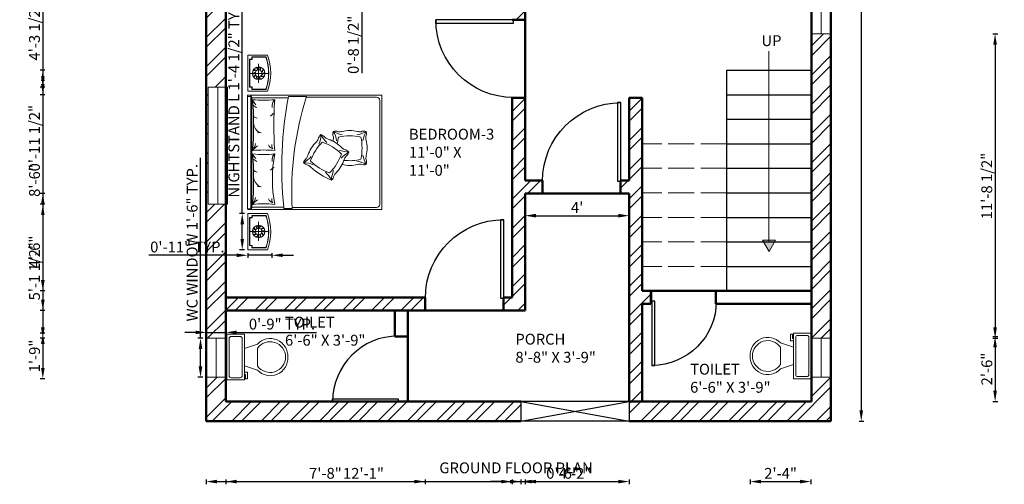
# Model space of a CAD drawing. Units: inches. Extents: x -83 to 371, y -457 to 76.
# Tile 1 of 4: x -83 to 371, y -457 to -243. Entities that reach past the tile are written whole.
import ezdxf

# ---------------------------------------------------------------- set-up
doc = ezdxf.new("R2010")
doc.units = ezdxf.units.IN
doc.linetypes.add('ACAD_ISO02W100', pattern=[15, 12, -3])
for name, color, linetype, lineweight in [('A-ANNO-DIMS', 2, 'Continuous', 18), ('A-ANNO-SYMB', 7, 'Continuous', 18), ('A-ANNO-TEXT', 7, 'Continuous', 25), ('A-AREA-IDEN', 7, 'Continuous', 25), ('A-DOOR', 3, 'Continuous', 25), ('A-FLOR-FIXT', 9, 'Continuous', 18), ('A-FLOR-STRS', 7, 'Continuous', 25), ('A-FLOR-STRS-OVHD', 8, 'ACAD_ISO02W100', 18), ('A-GLAZ', 4, 'Continuous', 18), ('A-WALL', 7, 'Continuous', 50), ('A-WALL-PATT', 252, 'Continuous', 13), ('furn', 28, 'Continuous', 18)]:
    doc.layers.add(name, color=color, linetype=linetype, lineweight=lineweight)
doc.styles.get("Standard").update_dxf_attribs({"font": 'arial.ttf'})
doc.dimstyles.new('ISO-25', dxfattribs={"dimtxt": 5, "dimasz": 5, "dimexe": 1.25, "dimexo": 0.625, "dimtad": 1, "dimlunit": 3, "dimtxsty": 'Standard', "dimcen": 2.5, "dimadec": 0, "dimazin": 0, "dimtfac": 1, "dimtmove": 0, "dimatfit": 3, "dimfxl": 1, "dimfxlon": 1, "dimarcsym": 0})

# ---------------------------------------------------------------- blocks, each defined once
blk = doc.blocks.new('*U2')
for p, q in [((9.5, -6), (9.5, -2)), ((-10, -8.5), (-8, -8.5)), ((-10, -9.5), (-10, -8.5)), ((-8, -8.5), (-8, -8)), ((-7, -8), (-7, -9.5)), ((-4, -8), (-6, -14)), ((4, -8), (6, -14)), ((-7, -9.5), (-10, -9.5)), ((4, -14), (-4, -14))]:
    blk.add_line(p, q)
blk.add_lwpolyline([(10.5, -8), (10.5, 0), (-10.5, 0), (-10.5, -8)], close=True)
for points in [[(-9.5, -2), (-9.5, -6)], [(8.5, -1), (-8.5, -1)], [(-8.5, -7), (8.5, -7)]]:
    blk.add_lwpolyline(points)
for centre, radius, start, end in [((-8.625, -1.875), 0.8839, 81.8699, 188.1301), ((8.625, -1.875), 0.8839, 351.8699, 98.1301), ((-8.625, -6.125), 0.8839, 171.869898, 278.1301), ((8.625, -6.125), 0.8839, 261.8699, 8.1301), ((-0.4772, -19.9188), 8.0953, 133.01722, 273.38), ((0.0374, -19.8731), 7.127, 124.50543, 269.7), ((-0.0373, -19.8731), 7.127, 270.3, 55.4946), ((0.4773, -19.9188), 8.0953, 266.62, 46.9828)]:
    blk.add_arc(centre, radius, start, end)
blk = doc.blocks.new('*U4')
for p, q in [((0, 0), (0, -6)), ((40, 0), (40, -6))]:
    blk.add_line(p, q)
blk.add_lwpolyline([(0, 0), (0, 40), (1.75, 40), (1.75, 0)], close=True)
blk.add_arc((0, 0), 40, 0, 90)
blk = doc.blocks.new('*D7')
at = {"layer": 'A-ANNO-DIMS', "color": 0, "lineweight": -2, "transparency": 16777216}
for p, q in [((149.97, -332.63), (149.97, -334.88)), ((154.97, -333.63), (192.97, -333.63)), ((197.97, -332.63), (197.97, -334.88))]:
    blk.add_line(p, q, dxfattribs=at)
at = {"layer": 'A-ANNO-DIMS', "color": 0, "transparency": 16777216}
for points in [[(154.97, -332.79), (154.97, -334.46), (149.97, -333.63)], [(192.97, -332.79), (192.97, -334.46), (197.97, -333.63)]]:
    blk.add_solid(points, dxfattribs=at)
at = {"layer": 'Defpoints', "color": 0, "transparency": 16777216}
for p in [(149.97, -331.2), (197.97, -331.2), (197.97, -333.63)]:
    blk.add_point(p, dxfattribs=at)
at = {"layer": 'A-ANNO-DIMS', "color": 0, "transparency": 16777216, "insert": (173.97, -330.5), "char_height": 5, "attachment_point": 5}
blk.add_mtext("4'", dxfattribs=at)
blk = doc.blocks.new('*D9')
at = {"layer": 'A-ANNO-DIMS', "color": 0, "lineweight": -2, "transparency": 16777216}
for p, q in [((303.95, 15.68), (306.2, 15.68)), ((304.95, 10.68), (304.95, -423.32)), ((303.95, -428.32), (306.2, -428.32))]:
    blk.add_line(p, q, dxfattribs=at)
at = {"layer": 'A-ANNO-DIMS', "color": 0, "transparency": 16777216}
for points in [[(304.12, 10.68), (305.78, 10.68), (304.95, 15.68)], [(304.12, -423.32), (305.78, -423.32), (304.95, -428.32)]]:
    blk.add_solid(points, dxfattribs=at)
at = {"layer": 'Defpoints', "color": 0, "transparency": 16777216}
for p in [(295.93, 15.68), (290.97, -428.32), (304.95, -428.32)]:
    blk.add_point(p, dxfattribs=at)
at = {"layer": 'A-ANNO-DIMS', "color": 0, "transparency": 16777216, "insert": (301.77, -206.32), "char_height": 5, "attachment_point": 5, "rotation": 90}
blk.add_mtext("37'", dxfattribs=at)
blk = doc.blocks.new('BED-DOUBLE')
for p, q in [((0.91, 59.91), (51.75, 59.91)), ((1.17, 60.37), (1.17, 45.16)), ((51.46, 60.37), (51.46, 43.19))]:
    blk.add_line(p, q)
for points in [[(0, 61.8), (0, 0), (52.66, 0), (52.66, 61.8)], [(52.17, 61.8), (52.17, 60.37), (0.3, 60.37), (0.3, 61.8), (52.66, 61.8)]]:
    blk.add_lwpolyline(points)
for points in [[(2.33, 49.32, 0.058596), (2.33, 59.5, 0.036889), (25.64, 59.5, 0.052163), (25.64, 49.32, 0.093111)], [(27.16, 49.32, 0.058596), (27.16, 59.5, 0.036648), (50.62, 59.5, 0.052163), (50.62, 49.32, 0.036967)], [(0.46, 45.16), (1.17, 45.16, -0.072944), (52.17, 43.04), (52.17, 34.6, 0.092568), (0.46, 41.29)]]:
    blk.add_lwpolyline(points, format="xyb", close=True)
for points in [[(0.91, 41.32), (0.91, 2.43, 0.414214), (2.43, 0.91), (50.23, 0.91, 0.414214), (51.75, 2.43), (51.75, 34.75)], [(16.91, 24, 0.111006), (25.6, 18.59, 0.119549), (31.09, 27.39, 0.107813), (22.42, 32.82)], [(22.37, 32.81, 0.121865), (16.91, 24, 0.121865)], [(20.68, 31.62, 0.091296), (21.61, 36.08, 0.091296), (24.41, 32.49, 0.091296)], [(26.47, 15.11, 0.159461), (27.65, 17.2, -0.076283), (28.59, 18.51, 0.115075), (32.41, 24.64, -0.076283), (33.17, 26.05, 0.159461), (34.52, 28.03)], [(30.07, 28.97, 0.091296), (34.52, 28.03, 0.091296), (30.93, 25.24, 0.091296)], [(18.01, 22.22, 0.091296), (13.56, 23.16, 0.091296), (17.15, 25.96, 0.091296)], [(23.17, 9.62, 0.111006), (33.41, 9.63, 0.119549), (33.41, 19.99, 0.033212), (30.26, 20.47)], [(27.4, 19.57, 0.091296), (26.47, 15.11, 0.091296), (23.67, 18.7)], [(31.71, 20.79, 0.091296), (35.99, 22.35, 0.091296), (34.42, 18.08, 0.091296)], [(35.99, 7.13, 0.159461), (35.88, 9.53, -0.076283), (35.99, 11.13, 0.115075), (35.99, 18.36, -0.076283), (35.88, 19.96, 0.159461), (35.99, 22.35)], [(25.05, 8.69, 0.091296), (20.77, 7.13, 0.091296), (22.34, 11.41, 0.091296)], [(34.42, 11.41, 0.091296), (35.99, 7.13, 0.091296), (31.71, 8.69)]]:
    blk.add_lwpolyline(points, format="xyb")
for centre, radius, start, end in [((0.91, 60.83), 0.913, 180, 270), ((7.74, 68), 10.08, 237.5379, 257.5233), ((-5.29, 49.98), 12.19, 36.4935, 51.2792), ((15.48, 53.46), 5.64, 96.6849, 148.3182), ((21.18, 56.67), 3.96, 141.8174, 169.8987), ((26.19, 56.11), 4.26, 130.5354, 160.3558), ((28.84, 52.52), 7.67, 114.6457, 134.1585), ((19.53, 49.98), 12.19, 36.4935, 51.2792), ((32.57, 68), 10.08, 237.5379, 257.5233), ((40.3, 53.46), 5.64, 96.6849, 148.3182), ((46.01, 56.67), 3.96, 141.8174, 169.8987), ((51.01, 56.11), 4.26, 130.5354, 160.3558), ((53.67, 52.52), 7.67, 114.6457, 134.1585), ((51.75, 60.83), 0.913, 270, 0), ((8.15, 56.6), 2.53, 335.8927, 16.1192), ((32.98, 56.6), 2.53, 335.8927, 16.1192), ((6.34, 49.09), 3.38, 114.2916, 160.9896), ((4.59, 48.38), 2.31, 76.4823, 128.5563), ((9.19, 42.25), 12.71, 36.2085, 45.0849), ((18.6, 49.75), 0.853, 353.7543, 77.2187), ((22.67, 46.41), 4.16, 44.406, 96.8342), ((23.45, 47.86), 2.64, 33.6349, 90.8456), ((31.17, 49.09), 3.38, 114.2916, 160.9896), ((29.41, 48.38), 2.31, 76.4823, 128.5563), ((34.02, 42.25), 12.71, 36.2085, 45.0849), ((43.42, 49.75), 0.853, 353.7543, 77.2187), ((47.5, 46.41), 4.16, 44.406, 96.8342), ((48.27, 47.86), 2.64, 33.6349, 90.8456), ((44.41, 10.55), 33.33, 138.3818, 157.7644), ((15.72, 36.39), 5.29, 315.5854, 333.0343), ((24.21, 33.23), 3.86, 132.4658, 168.7065), ((20.58, 32.5), 3.72, 37.2937, 74.0973), ((26.71, 38.99), 5.29, 233.2983, 250.7472), ((19.89, 18.93), 15.91, 45.1307, 71.3884), ((34.79, 33.99), 5.29, 225.7718, 243.2208), ((31.77, 25.77), 3.56, 39.4726, 79.6505), ((16.39, 25.78), 3.86, 222.6522, 258.8929), ((13.27, 17.27), 5.29, 45.7718, 63.2208), ((28.18, 32.33), 15.91, 225.1307, 251.3884), ((36.26, 14.74), 15.91, 166.8711, 193.1289), ((28.38, 6.89), 15.91, 77.0576, 78.7033), ((33.07, 27.55), 5.29, 257.6988, 275.1477), ((34.85, 18.98), 3.56, 71.3996, 111.5774), ((44.1, 14.85), 21.58, 173.1956, 194.0284), ((21.36, 12.27), 5.29, 53.2983, 70.7472), ((27.96, 19.27), 4.41, 218.7754, 250.3571), ((24.48, 8.17), 3.86, 159.3666, 195.6073), ((15.61, 9.99), 5.29, 355.0387, 12.4877), ((21.79, 10.85), 3.86, 254.5791, 290.8198), ((23.64, 1.98), 5.29, 77.6988, 95.1477), ((28.33, 22.65), 15.91, 257.0576, 283.3153), ((33.15, 2.01), 5.29, 85.2252, 102.6741), ((35.05, 11.45), 4.41, 250.7023, 282.284)]:
    blk.add_arc(centre, radius, start, end)
blk = doc.blocks.new('NIGHTSTAND-L')
for p, q in [((8.46, 1.22), (8.46, 10)), ((4.07, 5.61), (12.85, 5.61))]:
    blk.add_line(p, q)
blk.add_lwpolyline([(0, 1.52), (0, 10.65), (16.74, 10.65), (16.74, 1.52, -0.181818)], format="xyb", close=True)
for points in [[(1.92, 9.74), (1.92, 8.74), (0.91, 8.74)], [(2.01, 9.74), (2.01, 8.65), (0.91, 8.65)], [(1.92, 9.74), (14.83, 9.74)], [(1.92, 9.65), (14.83, 9.65)], [(14.73, 9.74), (14.73, 8.65), (15.83, 8.65)], [(14.83, 9.74), (14.83, 8.74), (15.83, 8.74)]]:
    blk.add_lwpolyline(points)
for points in [[(15.83, 8.74), (15.83, 2.16, -0.167087), (0.91, 2.16), (0.91, 8.74)], [(15.74, 8.74), (15.74, 2.22, -0.165559), (1, 2.22), (1, 8.74)]]:
    blk.add_lwpolyline(points, format="xyb")
for radius in [2.87, 1.55]:
    blk.add_circle((8.46, 5.61), radius)
for centre, radius, start, end in [((6.48, 6.34), 1.41, 232.3002, 292.538), ((6.49, 6.52), 1.84, 244.17, 290.4897), ((7.4, 7.5), 1.84, 208.17, 254.4897), ((7.28, 7.36), 1.41, 196.3002, 256.538), ((8.71, 7.76), 1.84, 172.17, 218.4897), ((8.53, 7.72), 1.41, 160.3002, 220.538), ((9.93, 7.2), 1.84, 136.17, 182.4897), ((9.76, 7.27), 1.41, 124.3002, 184.538), ((10.58, 6.04), 1.84, 100.17, 146.4897), ((10.49, 6.19), 1.41, 88.3002, 148.538), ((8.2, 3.47), 1.84, 352.17, 38.4897), ((10.42, 4.71), 1.84, 64.17, 110.4897), ((10.44, 4.89), 1.41, 52.3002, 112.538), ((9.64, 3.86), 1.41, 16.3002, 76.538), ((9.52, 3.73), 1.84, 28.17, 74.4897), ((6.43, 5.03), 1.41, 268.3002, 328.538), ((6.34, 5.19), 1.84, 280.17, 326.4897), ((7.16, 3.95), 1.41, 304.3002, 4.538), ((6.99, 4.02), 1.84, 316.17, 2.4897), ((8.38, 3.51), 1.41, 340.3002, 40.538)]:
    blk.add_arc(centre, radius, start, end)
blk = doc.blocks.new('NIGHTSTAND-R')
for p, q in [((8.28, 1.22), (8.28, 10)), ((12.67, 5.61), (3.89, 5.61))]:
    blk.add_line(p, q)
blk.add_lwpolyline([(16.74, 1.52), (16.74, 10.65), (0, 10.65), (0, 1.52, 0.181818)], format="xyb", close=True)
for points in [[(1.92, 9.74), (1.92, 8.74), (0.91, 8.74)], [(2.01, 9.74), (2.01, 8.65), (0.91, 8.65)], [(14.82, 9.74), (1.92, 9.74)], [(14.82, 9.65), (1.92, 9.65)], [(14.73, 9.74), (14.73, 8.65), (15.83, 8.65)], [(14.82, 9.74), (14.82, 8.74), (15.83, 8.74)]]:
    blk.add_lwpolyline(points)
for points in [[(0.91, 8.74), (0.91, 2.16, 0.167087), (15.83, 2.16), (15.83, 8.74)], [(1, 8.74), (1, 2.22, 0.165559), (15.74, 2.22), (15.74, 8.74)]]:
    blk.add_lwpolyline(points, format="xyb")
for radius in [2.87, 1.55]:
    blk.add_circle((8.28, 5.61), radius)
for centre, radius, start, end in [((6.3, 4.89), 1.41, 67.462, 127.6998), ((6.32, 4.7), 1.84, 69.5103, 115.83), ((7.23, 3.72), 1.84, 105.5103, 151.83), ((7.11, 3.86), 1.41, 103.462, 163.6998), ((6.26, 6.19), 1.41, 31.462, 91.6998), ((6.16, 6.03), 1.84, 33.5103, 79.83), ((8.54, 3.46), 1.84, 141.5103, 187.83), ((6.99, 7.27), 1.41, 355.462, 55.6998), ((6.82, 7.2), 1.84, 357.5103, 43.83), ((8.21, 7.72), 1.41, 319.462, 19.6998), ((8.24, 7.84), 1.84, 321.5103, 7.83), ((10.46, 6.59), 1.84, 249.5103, 295.83), ((10.48, 6.41), 1.41, 247.462, 307.6998), ((9.67, 7.44), 1.41, 283.462, 343.6998), ((9.55, 7.58), 1.84, 285.5103, 331.83), ((8.36, 3.5), 1.41, 139.462, 199.6998), ((9.75, 4.02), 1.84, 177.5103, 223.83), ((9.58, 3.95), 1.41, 175.462, 235.6998), ((10.41, 5.19), 1.84, 213.5103, 259.83), ((10.31, 5.03), 1.41, 211.462, 271.6998)]:
    blk.add_arc(centre, radius, start, end)
blk = doc.blocks.new('WIN-54IN')
blk.add_line((4.5, 54), (4.5, 0))
blk.add_lwpolyline([(0, 54), (9, 54), (9, 0), (0, 0)], close=True)
blk = doc.blocks.new('WIN-18IN')
blk.add_line((4.5, 18), (4.5, 0))
blk.add_lwpolyline([(0, 18), (9, 18), (9, 0), (0, 0)], close=True)
blk = doc.blocks.new('*D20')
at = {"layer": 'A-ANNO-DIMS', "color": 0, "lineweight": -2, "transparency": 16777216}
for p, q in [((0.34, -390.13), (0.34, -307.03)), ((1.34, -390.13), (-0.91, -390.13)), ((0.34, -403.13), (0.34, -395.13)), ((1.34, -408.13), (-0.91, -408.13))]:
    blk.add_line(p, q, dxfattribs=at)
at = {"layer": 'A-ANNO-DIMS', "color": 0, "transparency": 16777216}
for points in [[(-0.5, -395.13), (1.17, -395.13), (0.34, -390.13)], [(-0.5, -403.13), (1.17, -403.13), (0.34, -408.13)]]:
    blk.add_solid(points, dxfattribs=at)
at = {"layer": 'Defpoints', "color": 0, "transparency": 16777216}
for p in [(0.34, -390.13), (3.04, -390.13), (3.04, -408.13)]:
    blk.add_point(p, dxfattribs=at)
at = {"layer": 'A-ANNO-DIMS', "color": 0, "transparency": 16777216, "insert": (-2.87, -346.08), "char_height": 5, "attachment_point": 5, "rotation": 90}
blk.add_mtext('WC WINDOW 1\'-6" TYP.', dxfattribs=at)
blk = doc.blocks.new('*D21')
at = {"layer": 'A-ANNO-DIMS', "color": 0, "lineweight": -2, "transparency": 16777216}
for p, q in [((-1.96, -387.43), (-6.96, -387.43)), ((3.04, -388.43), (3.04, -386.18)), ((3.04, -387.43), (12.04, -387.43)), ((12.04, -388.43), (12.04, -386.18)), ((17.04, -387.43), (53.76, -387.43))]:
    blk.add_line(p, q, dxfattribs=at)
at = {"layer": 'A-ANNO-DIMS', "color": 0, "transparency": 16777216}
for points in [[(-1.96, -386.59), (-1.96, -388.26), (3.04, -387.43)], [(17.04, -386.59), (17.04, -388.26), (12.04, -387.43)]]:
    blk.add_solid(points, dxfattribs=at)
at = {"layer": 'Defpoints', "color": 0, "transparency": 16777216}
for p in [(3.04, -390.13), (12.04, -387.43), (12.04, -390.13)]:
    blk.add_point(p, dxfattribs=at)
at = {"layer": 'A-ANNO-DIMS', "color": 0, "transparency": 16777216, "insert": (37.9, -384.25), "char_height": 5, "attachment_point": 5}
blk.add_mtext('0\'-9" TYP.', dxfattribs=at)
blk = doc.blocks.new('*D24')
at = {"layer": 'A-ANNO-DIMS', "color": 0, "lineweight": -2, "transparency": 16777216}
for p, q in [((19.57, -332.63), (19.57, -231.32)), ((20.57, -332.63), (18.32, -332.63)), ((19.57, -344.37), (19.57, -337.63)), ((20.57, -349.37), (18.32, -349.37))]:
    blk.add_line(p, q, dxfattribs=at)
at = {"layer": 'A-ANNO-DIMS', "color": 0, "transparency": 16777216}
for points in [[(18.74, -337.63), (20.4, -337.63), (19.57, -332.63)], [(18.74, -344.37), (20.4, -344.37), (19.57, -349.37)]]:
    blk.add_solid(points, dxfattribs=at)
at = {"layer": 'Defpoints', "color": 0, "transparency": 16777216}
for p in [(19.57, -332.63), (22.08, -332.63), (22.08, -349.37)]:
    blk.add_point(p, dxfattribs=at)
at = {"layer": 'A-ANNO-DIMS', "color": 0, "transparency": 16777216, "insert": (16.36, -279.48), "char_height": 5, "attachment_point": 5, "rotation": 90}
blk.add_mtext('NIGHTSTAND L 1\'-4 1/2" TYP.', dxfattribs=at)
blk = doc.blocks.new('*D25')
at = {"layer": 'A-ANNO-DIMS', "color": 0, "lineweight": -2, "transparency": 16777216}
for p, q in [((17.08, -351.88), (-23.53, -351.88)), ((22.08, -350.88), (22.08, -353.13)), ((33.24, -351.88), (22.08, -351.88)), ((33.24, -350.88), (33.24, -353.13)), ((38.24, -351.88), (43.24, -351.88))]:
    blk.add_line(p, q, dxfattribs=at)
at = {"layer": 'A-ANNO-DIMS', "color": 0, "transparency": 16777216}
for points in [[(17.08, -351.05), (17.08, -352.71), (22.08, -351.88)], [(38.24, -351.05), (38.24, -352.71), (33.24, -351.88)]]:
    blk.add_solid(points, dxfattribs=at)
at = {"layer": 'Defpoints', "color": 0, "transparency": 16777216}
for p in [(22.08, -349.37), (33.24, -349.37), (22.08, -351.88)]:
    blk.add_point(p, dxfattribs=at)
at = {"layer": 'A-ANNO-DIMS', "color": 0, "transparency": 16777216, "insert": (-5.72, -348.7), "char_height": 5, "attachment_point": 5}
blk.add_mtext('0\'-11" TYP.', dxfattribs=at)
blk = doc.blocks.new('*D37')
at = {"layer": 'A-ANNO-DIMS', "color": 0, "lineweight": -2, "transparency": 16777216}
for p, q in [((74.66, -218.28), (74.66, -213.28)), ((73.66, -223.28), (75.91, -223.28)), ((74.66, -223.28), (74.66, -231.78)), ((73.66, -231.78), (75.91, -231.78)), ((74.66, -236.78), (74.66, -267.97))]:
    blk.add_line(p, q, dxfattribs=at)
at = {"layer": 'A-ANNO-DIMS', "color": 0, "transparency": 16777216}
for points in [[(73.83, -218.28), (75.5, -218.28), (74.66, -223.28)], [(73.83, -236.78), (75.5, -236.78), (74.66, -231.78)]]:
    blk.add_solid(points, dxfattribs=at)
at = {"layer": 'Defpoints', "color": 0, "transparency": 16777216}
for p in [(72.86, -223.28), (72.86, -231.78), (74.66, -231.78)]:
    blk.add_point(p, dxfattribs=at)
at = {"layer": 'A-ANNO-DIMS', "color": 0, "transparency": 16777216, "insert": (71.45, -254.88), "char_height": 5, "attachment_point": 5, "rotation": 90}
blk.add_mtext('0\'-8 1/2"', dxfattribs=at)
blk = doc.blocks.new('*D40')
at = {"layer": 'A-ANNO-DIMS', "color": 0, "lineweight": -2, "transparency": 16777216}
for p, q in [((-71.36, -222.99), (-73.61, -222.99)), ((-72.36, -227.99), (-72.36, -269.39)), ((-71.36, -274.39), (-73.61, -274.39))]:
    blk.add_line(p, q, dxfattribs=at)
at = {"layer": 'A-ANNO-DIMS', "color": 0, "transparency": 16777216}
for points in [[(-73.19, -227.99), (-71.52, -227.99), (-72.36, -222.99)], [(-73.19, -269.39), (-71.52, -269.39), (-72.36, -274.39)]]:
    blk.add_solid(points, dxfattribs=at)
at = {"layer": 'Defpoints', "color": 0, "transparency": 16777216}
for p in [(3.06, -222.99), (-72.36, -274.39), (3.85, -274.39)]:
    blk.add_point(p, dxfattribs=at)
at = {"layer": 'A-ANNO-DIMS', "color": 0, "transparency": 16777216, "insert": (-75.57, -248.69), "char_height": 5, "attachment_point": 5, "rotation": 90}
blk.add_mtext('4\'-3 1/2"', dxfattribs=at)
blk = doc.blocks.new('*D41')
at = {"layer": 'A-ANNO-DIMS', "color": 0, "lineweight": -2, "transparency": 16777216}
for p, q in [((-71.36, -328.39), (-73.61, -328.39)), ((-72.36, -333.39), (-72.36, -385.13)), ((-71.36, -390.13), (-73.61, -390.13))]:
    blk.add_line(p, q, dxfattribs=at)
at = {"layer": 'A-ANNO-DIMS', "color": 0, "transparency": 16777216}
for points in [[(-73.19, -333.39), (-71.52, -333.39), (-72.36, -328.39)], [(-73.19, -385.13), (-71.52, -385.13), (-72.36, -390.13)]]:
    blk.add_solid(points, dxfattribs=at)
at = {"layer": 'Defpoints', "color": 0, "transparency": 16777216}
for p in [(3.85, -328.39), (-72.36, -390.13), (3.04, -390.13)]:
    blk.add_point(p, dxfattribs=at)
at = {"layer": 'A-ANNO-DIMS', "color": 0, "transparency": 16777216, "insert": (-75.57, -359.26), "char_height": 5, "attachment_point": 5, "rotation": 90}
blk.add_mtext('5\'-1 1/2"', dxfattribs=at)
blk = doc.blocks.new('*D44')
at = {"layer": 'A-ANNO-DIMS', "color": 0, "lineweight": -2, "transparency": 16777216}
for p, q in [((365.66, -249.79), (367.91, -249.79)), ((366.66, -254.79), (366.66, -385.13)), ((365.66, -390.13), (367.91, -390.13))]:
    blk.add_line(p, q, dxfattribs=at)
at = {"layer": 'A-ANNO-DIMS', "color": 0, "transparency": 16777216}
for points in [[(365.83, -254.79), (367.49, -254.79), (366.66, -249.79)], [(365.83, -385.13), (367.49, -385.13), (366.66, -390.13)]]:
    blk.add_solid(points, dxfattribs=at)
at = {"layer": 'Defpoints', "color": 0, "transparency": 16777216}
for p in [(290.97, -249.79), (290.97, -390.13), (366.66, -390.13)]:
    blk.add_point(p, dxfattribs=at)
at = {"layer": 'A-ANNO-DIMS', "color": 0, "transparency": 16777216, "insert": (363.45, -319.96), "char_height": 5, "attachment_point": 5, "rotation": 90}
blk.add_mtext('11\'-8 1/2"', dxfattribs=at)
blk = doc.blocks.new('*D45')
at = {"layer": 'A-ANNO-DIMS', "color": 0, "lineweight": -2, "transparency": 16777216}
for p, q in [((138.97, -456.2), (133.97, -456.2)), ((143.97, -455.2), (143.97, -457.45)), ((143.97, -456.2), (149.97, -456.2)), ((149.97, -455.2), (149.97, -457.45)), ((154.97, -456.2), (174.51, -456.2))]:
    blk.add_line(p, q, dxfattribs=at)
at = {"layer": 'A-ANNO-DIMS', "color": 0, "transparency": 16777216}
for points in [[(138.97, -455.37), (138.97, -457.03), (143.97, -456.2)], [(154.97, -455.37), (154.97, -457.03), (149.97, -456.2)]]:
    blk.add_solid(points, dxfattribs=at)
at = {"layer": 'Defpoints', "color": 0, "transparency": 16777216}
for p in [(143.97, 6.68), (149.97, 6.68), (149.97, -456.2)]:
    blk.add_point(p, dxfattribs=at)
at = {"layer": 'A-ANNO-DIMS', "color": 0, "transparency": 16777216, "insert": (167.24, -453.02), "char_height": 5, "attachment_point": 5}
blk.add_mtext('0\'-6"', dxfattribs=at)
blk = doc.blocks.new('*D48')
at = {"layer": 'A-ANNO-DIMS', "color": 0, "lineweight": -2, "transparency": 16777216}
for p, q in [((242.97, 39.58), (242.97, 41.83)), ((281.97, 39.58), (281.97, 41.83)), ((247.97, 40.58), (276.97, 40.58))]:
    blk.add_line(p, q, dxfattribs=at)
at = {"layer": 'A-ANNO-DIMS', "color": 0, "transparency": 16777216}
for points in [[(247.97, 41.41), (247.97, 39.74), (242.97, 40.58)], [(276.97, 41.41), (276.97, 39.74), (281.97, 40.58)]]:
    blk.add_solid(points, dxfattribs=at)
at = {"layer": 'Defpoints', "color": 0, "transparency": 16777216}
for p in [(281.97, 40.58), (242.97, -266.56), (281.97, -266.56)]:
    blk.add_point(p, dxfattribs=at)
at = {"layer": 'A-ANNO-DIMS', "color": 0, "transparency": 16777216, "insert": (262.47, 43.75), "char_height": 5, "attachment_point": 5}
blk.add_mtext('3\'-3"', dxfattribs=at)
blk = doc.blocks.new('*D49')
at = {"layer": 'A-ANNO-DIMS', "color": 0, "lineweight": -2, "transparency": 16777216}
for p, q in [((-71.36, -266.56), (-73.61, -266.56)), ((-72.36, -271.56), (-72.36, -272.87)), ((-71.36, -277.87), (-73.61, -277.87)), ((-72.36, -277.87), (-72.36, -312.95))]:
    blk.add_line(p, q, dxfattribs=at)
at = {"layer": 'A-ANNO-DIMS', "color": 0, "transparency": 16777216}
for points in [[(-73.19, -271.56), (-71.52, -271.56), (-72.36, -266.56)], [(-73.19, -272.87), (-71.52, -272.87), (-72.36, -277.87)]]:
    blk.add_solid(points, dxfattribs=at)
at = {"layer": 'Defpoints', "color": 0, "transparency": 16777216}
for p in [(242.97, -266.56), (-72.36, -277.87), (242.97, -277.87)]:
    blk.add_point(p, dxfattribs=at)
at = {"layer": 'A-ANNO-DIMS', "color": 0, "transparency": 16777216, "insert": (-75.57, -297.91), "char_height": 5, "attachment_point": 5, "rotation": 90}
blk.add_mtext('0\'-11 1/2"', dxfattribs=at)
blk = doc.blocks.new('*D50')
at = {"layer": 'A-ANNO-DIMS', "color": 0, "lineweight": -2, "transparency": 16777216}
for p, q in [((-71.36, -266.56), (-73.61, -266.56)), ((-72.36, -271.56), (-72.36, -363.32)), ((-71.36, -368.32), (-73.61, -368.32))]:
    blk.add_line(p, q, dxfattribs=at)
at = {"layer": 'A-ANNO-DIMS', "color": 0, "transparency": 16777216}
for points in [[(-73.19, -271.56), (-71.52, -271.56), (-72.36, -266.56)], [(-73.19, -363.32), (-71.52, -363.32), (-72.36, -368.32)]]:
    blk.add_solid(points, dxfattribs=at)
at = {"layer": 'Defpoints', "color": 0, "transparency": 16777216}
for p in [(281.97, -266.56), (-72.36, -368.32), (281.97, -368.32)]:
    blk.add_point(p, dxfattribs=at)
at = {"layer": 'A-ANNO-DIMS', "color": 0, "transparency": 16777216, "insert": (-75.54, -317.44), "char_height": 5, "attachment_point": 5, "rotation": 90}
blk.add_mtext('8\'-6"', dxfattribs=at)
blk = doc.blocks.new('*D51')
at = {"layer": 'A-ANNO-DIMS', "color": 0, "lineweight": -2, "transparency": 16777216}
for p, q in [((2.97, -455.2), (2.97, -457.45)), ((7.97, -456.2), (142.97, -456.2)), ((147.97, -455.2), (147.97, -457.45))]:
    blk.add_line(p, q, dxfattribs=at)
at = {"layer": 'A-ANNO-DIMS', "color": 0, "transparency": 16777216}
for points in [[(7.97, -455.37), (7.97, -457.03), (2.97, -456.2)], [(142.97, -455.37), (142.97, -457.03), (147.97, -456.2)]]:
    blk.add_solid(points, dxfattribs=at)
at = {"layer": 'Defpoints', "color": 0, "transparency": 16777216}
for p in [(2.97, -428.32), (147.97, -428.32), (147.97, -456.2)]:
    blk.add_point(p, dxfattribs=at)
at = {"layer": 'A-ANNO-DIMS', "color": 0, "transparency": 16777216, "insert": (75.47, -453.06), "char_height": 5, "attachment_point": 5}
blk.add_mtext('12\'-1"', dxfattribs=at)
blk = doc.blocks.new('*D52')
at = {"layer": 'A-ANNO-DIMS', "color": 0, "lineweight": -2, "transparency": 16777216}
for p, q in [((147.97, -455.2), (147.97, -457.45)), ((152.97, -456.2), (192.97, -456.2)), ((197.97, -455.2), (197.97, -457.45))]:
    blk.add_line(p, q, dxfattribs=at)
at = {"layer": 'A-ANNO-DIMS', "color": 0, "transparency": 16777216}
for points in [[(152.97, -455.37), (152.97, -457.03), (147.97, -456.2)], [(192.97, -455.37), (192.97, -457.03), (197.97, -456.2)]]:
    blk.add_solid(points, dxfattribs=at)
at = {"layer": 'Defpoints', "color": 0, "transparency": 16777216}
for p in [(147.97, -428.32), (197.97, -428.32), (197.97, -456.2)]:
    blk.add_point(p, dxfattribs=at)
at = {"layer": 'A-ANNO-DIMS', "color": 0, "transparency": 16777216, "insert": (172.97, -453.06), "char_height": 5, "attachment_point": 5}
blk.add_mtext('4\'-2"', dxfattribs=at)
blk = doc.blocks.new('*D53')
at = {"layer": 'A-ANNO-DIMS', "color": 0, "lineweight": -2, "transparency": 16777216}
for p, q in [((-71.36, -323.37), (-73.61, -323.37)), ((-72.36, -328.37), (-72.36, -372.32)), ((-71.36, -377.32), (-73.61, -377.32))]:
    blk.add_line(p, q, dxfattribs=at)
at = {"layer": 'A-ANNO-DIMS', "color": 0, "transparency": 16777216}
for points in [[(-73.19, -328.37), (-71.52, -328.37), (-72.36, -323.37)], [(-73.19, -372.32), (-71.52, -372.32), (-72.36, -377.32)]]:
    blk.add_solid(points, dxfattribs=at)
at = {"layer": 'Defpoints', "color": 0, "transparency": 16777216}
for p in [(149.97, -323.37), (-72.36, -377.32), (149.97, -377.32)]:
    blk.add_point(p, dxfattribs=at)
at = {"layer": 'A-ANNO-DIMS', "color": 0, "transparency": 16777216, "insert": (-75.54, -350.35), "char_height": 5, "attachment_point": 5, "rotation": 90}
blk.add_mtext('4\'-6"', dxfattribs=at)
blk = doc.blocks.new('*D54')
at = {"layer": 'A-ANNO-DIMS', "color": 0, "lineweight": -2, "transparency": 16777216}
for p, q in [((365.66, -389.32), (367.91, -389.32)), ((366.66, -394.32), (366.66, -414.32)), ((365.66, -419.32), (367.91, -419.32))]:
    blk.add_line(p, q, dxfattribs=at)
at = {"layer": 'A-ANNO-DIMS', "color": 0, "transparency": 16777216}
for points in [[(365.83, -394.32), (367.49, -394.32), (366.66, -389.32)], [(365.83, -414.32), (367.49, -414.32), (366.66, -419.32)]]:
    blk.add_solid(points, dxfattribs=at)
at = {"layer": 'Defpoints', "color": 0, "transparency": 16777216}
for p in [(95.97, -389.32), (95.97, -419.32), (366.66, -419.32)]:
    blk.add_point(p, dxfattribs=at)
at = {"layer": 'A-ANNO-DIMS', "color": 0, "transparency": 16777216, "insert": (363.48, -404.32), "char_height": 5, "attachment_point": 5, "rotation": 90}
blk.add_mtext('2\'-6"', dxfattribs=at)
blk = doc.blocks.new('*D55')
at = {"layer": 'A-ANNO-DIMS', "color": 0, "lineweight": -2, "transparency": 16777216}
for p, q in [((11.97, -455.2), (11.97, -457.45)), ((16.97, -456.2), (98.87, -456.2)), ((103.87, -455.2), (103.87, -457.45))]:
    blk.add_line(p, q, dxfattribs=at)
at = {"layer": 'A-ANNO-DIMS', "color": 0, "transparency": 16777216}
for points in [[(16.97, -455.37), (16.97, -457.03), (11.97, -456.2)], [(98.87, -455.37), (98.87, -457.03), (103.87, -456.2)]]:
    blk.add_solid(points, dxfattribs=at)
at = {"layer": 'Defpoints', "color": 0, "transparency": 16777216}
for p in [(11.97, -233.32), (103.87, -233.32), (103.87, -456.2)]:
    blk.add_point(p, dxfattribs=at)
at = {"layer": 'A-ANNO-DIMS', "color": 0, "transparency": 16777216, "insert": (57.92, -453.02), "char_height": 5, "attachment_point": 5}
blk.add_mtext('7\'-8"', dxfattribs=at)
blk = doc.blocks.new('*D63')
at = {"layer": 'A-ANNO-DIMS', "color": 0, "lineweight": -2, "transparency": 16777216}
for p, q in [((253.76, -455.2), (253.76, -457.45)), ((258.76, -456.2), (276.76, -456.2)), ((281.76, -455.2), (281.76, -457.45))]:
    blk.add_line(p, q, dxfattribs=at)
at = {"layer": 'A-ANNO-DIMS', "color": 0, "transparency": 16777216}
for points in [[(258.76, -455.37), (258.76, -457.03), (253.76, -456.2)], [(276.76, -455.37), (276.76, -457.03), (281.76, -456.2)]]:
    blk.add_solid(points, dxfattribs=at)
at = {"layer": 'Defpoints', "color": 0, "transparency": 16777216}
for p in [(253.76, -398.3), (281.76, -408.8), (281.76, -456.2)]:
    blk.add_point(p, dxfattribs=at)
at = {"layer": 'A-ANNO-DIMS', "color": 0, "transparency": 16777216, "insert": (267.76, -453.06), "char_height": 5, "attachment_point": 5}
blk.add_mtext('2\'-4"', dxfattribs=at)
blk = doc.blocks.new('*D64')
at = {"layer": 'A-ANNO-DIMS', "color": 0, "lineweight": -2, "transparency": 16777216}
for p, q in [((-71.36, -387.8), (-73.61, -387.8)), ((-72.36, -392.8), (-72.36, -403.8)), ((-71.36, -408.8), (-73.61, -408.8))]:
    blk.add_line(p, q, dxfattribs=at)
at = {"layer": 'A-ANNO-DIMS', "color": 0, "transparency": 16777216}
for points in [[(-73.19, -392.8), (-71.52, -392.8), (-72.36, -387.8)], [(-73.19, -403.8), (-71.52, -403.8), (-72.36, -408.8)]]:
    blk.add_solid(points, dxfattribs=at)
at = {"layer": 'Defpoints', "color": 0, "transparency": 16777216}
for p in [(273.76, -387.8), (-72.36, -408.8), (273.76, -408.8)]:
    blk.add_point(p, dxfattribs=at)
at = {"layer": 'A-ANNO-DIMS', "color": 0, "transparency": 16777216, "insert": (-75.54, -398.3), "char_height": 5, "attachment_point": 5, "rotation": 90}
blk.add_mtext('1\'-9"', dxfattribs=at)

msp = doc.modelspace()

# ---------------------------------------------------------------- hatches: boundary and pattern name
at = {"layer": 'A-ANNO-SYMB'}
h = msp.add_hatch(color=256, dxfattribs=at)
h.dxf.hatch_style = 1
h.paths.add_polyline_path([(262.451, -350.19), (265.451, -344.994), (259.451, -344.994)])
at = {"layer": 'A-WALL-PATT'}
h = msp.add_hatch(dxfattribs=at)
h.set_pattern_fill('ANSI32', color=256)
h.set_pattern_definition([(45, (-445.966, 5e-14), (-6.73519, 6.73519), []), (45, (-441.476, 5e-14), (-6.73519, 6.73519), [])])
h.paths.add_polyline_path([(147.969, -419.325), (11.969, -419.325), (11.969, -408.128), (2.969, -408.128), (2.969, -428.325), (147.969, -428.325)])
h.paths.add_polyline_path([(290.969, -408.128), (281.969, -408.128), (281.969, -419.325), (197.969, -419.325), (197.969, -428.325), (290.969, -428.325)])
h.paths.add_polyline_path([(203.969, -374.325), (207.969, -374.325), (207.969, -368.325), (203.969, -368.325), (203.969, -279.294), (197.969, -279.294), (197.969, -317.37), (194.142, -317.37), (194.142, -317.678), (194.142, -323.37), (197.969, -323.37), (197.969, -374.325), (197.969, -419.325), (203.969, -419.325)])
h.paths.add_polyline_path([(290.969, -249.793), (281.969, -249.793), (281.969, -390.128), (290.969, -390.128)])
h.paths.add_polyline_path([(149.969, -323.37), (157.969, -323.37), (157.969, -317.37), (149.969, -317.37), (149.969, -279.294), (143.969, -279.294), (143.969, -371.325), (140.142, -371.325), (140.142, -371.632), (140.142, -377.325), (143.969, -377.325), (149.969, -377.325)])
h.paths.add_polyline_path([(103.969, -371.325), (11.969, -371.325), (11.969, -377.325), (103.969, -377.325)])
h.paths.add_polyline_path([(11.969, -328.391), (3.855, -328.391), (3.855, -274.391), (11.969, -274.391), (11.969, -222.986), (2.969, -222.986), (2.969, -390.128), (11.969, -390.128)])
h.paths.add_polyline_path([(149.969, -233.325), (143.969, -233.325), (11.969, -233.325), (11.969, -239.325), (143.969, -239.325), (143.969, -243.294), (144.688, -243.294), (149.969, -243.294)])
h.paths.add_polyline_path([(11.969, -86.501), (2.969, -86.501), (2.969, -168.986), (11.969, -168.986)])
h.paths.add_polyline_path([(103.969, -149.325), (11.969, -149.325), (11.969, -155.325), (103.969, -155.325)])
h.paths.add_polyline_path([(149.969, 6.675), (143.969, 6.675), (143.969, -149.325), (139.969, -149.325), (139.969, -155.325), (153.969, -155.325), (153.969, -149.325), (149.969, -149.325)])
h.paths.add_polyline_path([(281.969, -149.325), (189.973, -149.325, -0.0041567), (189.978, -149.923), (189.978, -155.325), (281.969, -155.325)])
h.paths.add_polyline_path([(290.969, -90.886), (281.969, -90.886), (281.969, -195.793), (290.969, -195.793)])
h.paths.add_polyline_path([(290.969, 15.675), (2.969, 15.675), (2.969, -32.501), (11.969, -32.501), (11.969, 6.675), (281.969, 6.675), (281.969, -36.886), (290.969, -36.886)])

# ---------------------------------------------------------------- linework, layer by layer
at = {"layer": 'A-ANNO-SYMB'}
msp.add_line((262.413, -257.755), (262.413, -345.711), dxfattribs=at)
msp.add_lwpolyline([(262.451, -350.19), (265.451, -344.994), (259.451, -344.994), (262.451, -350.19)], dxfattribs=at)
at = {"layer": 'A-DOOR'}
for p, q in [((147.969, -419.325), (147.969, -428.325)), ((197.969, -419.325), (147.969, -419.325)), ((147.969, -428.325), (197.969, -419.325)), ((147.969, -419.325), (197.969, -428.325)), ((197.969, -419.325), (197.969, -428.325)), ((197.969, -428.325), (147.969, -428.325))]:
    msp.add_line(p, q, dxfattribs=at)
at = {"layer": 'A-FLOR-STRS'}
for p, q in [((242.969, -368.325), (242.969, -266.561)), ((242.969, -266.561), (281.969, -266.561)), ((242.969, -277.868), (281.969, -277.868)), ((242.969, -289.175), (281.969, -289.175)), ((242.969, -300.482), (281.969, -300.482)), ((242.969, -311.79), (281.969, -311.79)), ((242.969, -323.097), (281.969, -323.097)), ((242.969, -334.404), (281.969, -334.404)), ((242.969, -345.711), (281.969, -345.711)), ((242.969, -357.018), (281.969, -357.018)), ((242.969, -368.325), (281.969, -368.325))]:
    msp.add_line(p, q, dxfattribs=at)
at = {"layer": 'A-FLOR-STRS-OVHD'}
for p, q in [((242.969, -300.482), (203.969, -300.482)), ((242.969, -311.79), (203.969, -311.79)), ((242.969, -323.097), (203.969, -323.097)), ((242.969, -334.404), (203.969, -334.404)), ((242.969, -345.711), (203.969, -345.711)), ((242.969, -357.018), (203.969, -357.018)), ((242.969, -368.325), (203.969, -368.325))]:
    msp.add_line(p, q, dxfattribs=at)
at = {"layer": 'A-WALL'}
for p, q in [((2.969, -428.325), (2.969, 15.675)), ((290.969, 15.675), (290.969, -428.325)), ((11.969, -419.325), (11.969, 6.675)), ((281.969, 6.675), (281.969, -419.325)), ((149.969, -317.37), (149.969, -233.325)), ((143.969, -243.294), (149.969, -243.294)), ((143.969, -371.325), (143.969, -279.294)), ((143.969, -279.294), (149.969, -279.294)), ((197.969, -279.294), (203.969, -279.294)), ((197.969, -317.37), (197.969, -279.294)), ((203.969, -279.294), (203.969, -368.325)), ((157.969, -317.37), (149.969, -317.37)), ((157.969, -317.37), (157.969, -323.37)), ((197.969, -317.37), (193.969, -317.37)), ((193.969, -317.37), (193.969, -323.37)), ((149.969, -377.325), (149.969, -323.37)), ((193.969, -323.37), (149.969, -323.37)), ((193.969, -323.37), (197.969, -323.37)), ((197.969, -374.325), (197.969, -323.37)), ((103.969, -371.325), (11.969, -371.325)), ((103.969, -371.325), (103.969, -377.325)), ((143.969, -371.325), (139.969, -371.325)), ((139.969, -371.325), (139.969, -377.325)), ((203.969, -368.325), (281.969, -368.325)), ((207.969, -374.325), (207.969, -368.325)), ((237.969, -374.325), (237.969, -368.325)), ((197.969, -419.325), (197.969, -374.325)), ((203.969, -419.325), (203.969, -374.325)), ((203.969, -374.325), (207.969, -374.325)), ((237.969, -374.325), (281.969, -374.325)), ((143.969, -377.325), (11.969, -377.325)), ((89.969, -389.325), (89.969, -377.325)), ((95.969, -419.325), (95.969, -377.325)), ((143.969, -377.325), (149.969, -377.325)), ((95.969, -389.325), (89.969, -389.325)), ((147.969, -419.325), (11.969, -419.325)), ((281.969, -419.325), (197.969, -419.325)), ((147.969, -428.325), (2.969, -428.325)), ((290.969, -428.325), (197.969, -428.325))]:
    msp.add_line(p, q, dxfattribs=at)

# ---------------------------------------------------------------- block references
at = {"layer": 'A-DOOR'}
for p, xscale, yscale, zscale, rotation in [((144.688, -243.294), -0.8974971094035348, 0.8974971094035348, 0.8974971094035348, 90), ((208.47, -372.968), -0.7417545504100413, 0.7417545504100413, 0.7417545504100413, 180), ((91.437, -419.327), 0.7554361559037658, 0.7554361559037658, 0.7554361559037658, 90)]:
    msp.add_blockref('*U4', p, dxfattribs=dict(at, xscale=xscale, yscale=yscale, zscale=zscale, rotation=rotation))
at = {"layer": 'A-DOOR', "xscale": -0.9035591955078199, "yscale": 0.9035591955078199, "zscale": 0.9035591955078199}
for p in [(194.142, -317.678), (140.142, -371.632)]:
    msp.add_blockref('*U4', p, dxfattribs=at)
at = {"layer": 'A-FLOR-FIXT'}
for p, rotation in [((12.542, -398.819), 90), ((281.759, -398.3), 270)]:
    msp.add_blockref('*U2', p, dxfattribs=dict(at, rotation=rotation))
at = {"layer": 'A-GLAZ'}
for name, p in [('WIN-54IN', (281.969, -249.792)), ('WIN-54IN', (3.854, -328.39)), ('WIN-18IN', (3.037, -408.128)), ('WIN-18IN', (281.969, -408.128))]:
    msp.add_blockref(name, p, dxfattribs=at)
at = {"layer": 'furn'}
for name, p, rotation in [('NIGHTSTAND-R', (32.734, -276.31), 90.00000000000021), ('BED-DOUBLE', (83.874, -330.8), 89.99999999999996), ('NIGHTSTAND-L', (32.737, -349.37), 89.99999999999888)]:
    msp.add_blockref(name, p, dxfattribs=dict(at, rotation=rotation))

# ---------------------------------------------------------------- texts
at = {"layer": 'A-ANNO-TEXT', "char_height": 5, "attachment_point": 1}
for s, width, insert in [('UP', 11.75896, (258.942, -250.471)), ('GROUND FLOOR PLAN', 260.85029, (110.437, -447.367))]:
    msp.add_mtext_dynamic_manual_height_columns(s, width=width, gutter_width=12.5, heights=[0], dxfattribs=dict(at, insert=insert))
at = {"layer": 'A-AREA-IDEN', "char_height": 5, "attachment_point": 1}
for s, width, insert in [('BEDROOM-3\\P11\'-0" X 11\'-0"', 44.31167, (96.41, -293.567)), ('TOILET\\P6\'-6" X 3\'-9"', 43.44671, (39.278, -380.201)), ('PORCH\\P8\'-8" X 3\'-9"', 37.54632, (145.503, -388.056)), ('TOILET\\P6\'-6" X 3\'-9"', 41.70155, (226.048, -401.897))]:
    msp.add_mtext_dynamic_manual_height_columns(s, width=width, gutter_width=12.5, heights=[0], dxfattribs=dict(at, insert=insert))

# ---------------------------------------------------------------- dimensions: what is measured, and where the dimension line sits
at = {"layer": 'A-ANNO-DIMS'}
for base, p1, p2, override, picture, middle in [((281.969, 40.575), (242.969, -266.561), (281.969, -266.561), {"dimdec": 1, "dimlfac": 1, "dimrnd": 0, "dimzin": 1, "dimdsep": 46, "dimlunit": 4, "dimfrac": 2}, '*D48', (262.469, 43.755)), ((149.969, -456.2), (143.969, 6.675), (149.969, 6.675), {"dimdec": 1, "dimlfac": 1, "dimrnd": 0, "dimzin": 1, "dimdsep": 46, "dimlunit": 4, "dimfrac": 2}, '*D45', (167.24, -453.022)), ((103.866, -456.2), (11.969, -233.325), (103.866, -233.325), {"dimdec": 1, "dimlfac": 1, "dimrnd": 0, "dimzin": 1, "dimdsep": 46, "dimlunit": 4, "dimfrac": 2}, '*D55', (57.917, -453.022)), ((197.969, -333.627), (149.969, -331.197), (197.969, -331.197), {"dimclrd": 0, "dimclre": 0, "dimclrt": 0}, '*D7', (173.969, -330.502)), ((281.759, -456.2), (253.759, -398.3), (281.759, -408.8), {"dimdec": 1, "dimlfac": 1, "dimrnd": 0, "dimzin": 1, "dimdsep": 46, "dimlunit": 4, "dimfrac": 2}, '*D63', (267.759, -453.065)), ((147.969, -456.2), (2.969, -428.325), (147.969, -428.325), {"dimdec": 1, "dimlfac": 1, "dimrnd": 0, "dimzin": 1, "dimdsep": 46, "dimlunit": 4, "dimfrac": 2}, '*D51', (75.469, -453.065)), ((197.969, -456.2), (147.969, -428.325), (197.969, -428.325), {"dimdec": 1, "dimlfac": 1, "dimrnd": 0, "dimzin": 1, "dimdsep": 46, "dimlunit": 4, "dimfrac": 2}, '*D52', (172.969, -453.065))]:
    dim = msp.add_linear_dim(base=base, p1=p1, p2=p2, dimstyle='ISO-25', override=override, dxfattribs=at)
    dim.commit()
    dim.dimension.update_dxf_attribs({"geometry": picture, "text_midpoint": middle})
for base, p1, p2, angle, override, picture, middle in [((304.949, -428.325), (295.93, 15.675), (290.969, -428.325), 90, {"dimclrd": 0, "dimclre": 0, "dimclrt": 0}, '*D9', (301.769, -206.325)), ((74.663, -231.78), (72.863, -223.281), (72.863, -231.78), 270, {"dimdec": 1, "dimlfac": 1, "dimrnd": 0, "dimzin": 1, "dimdsep": 46, "dimlunit": 4, "dimfrac": 2}, '*D37', (71.453, -254.876)), ((-72.358, -274.391), (3.062, -222.986), (3.855, -274.391), 90, {"dimdec": 1, "dimlfac": 1, "dimrnd": 0, "dimzin": 1, "dimdsep": 46, "dimlunit": 4, "dimfrac": 2}, '*D40', (-75.57, -248.688)), ((366.659, -390.128), (290.969, -249.793), (290.969, -390.128), 90, {"dimdec": 1, "dimlfac": 1, "dimrnd": 0, "dimzin": 1, "dimdsep": 46, "dimlunit": 4, "dimfrac": 2}, '*D44', (363.448, -319.96)), ((-72.358, -277.868), (242.969, -266.561), (242.969, -277.868), 90, {"dimdec": 1, "dimlfac": 1, "dimrnd": 0, "dimzin": 1, "dimdsep": 46, "dimlunit": 4, "dimfrac": 2}, '*D49', (-75.568, -297.907)), ((-72.358, -368.325), (281.969, -266.561), (281.969, -368.325), 90, {"dimdec": 1, "dimlfac": 1, "dimrnd": 0, "dimzin": 1, "dimdsep": 46, "dimlunit": 4, "dimfrac": 2}, '*D50', (-75.536, -317.443)), ((-72.358, -377.325), (149.969, -323.37), (149.969, -377.325), 90, {"dimdec": 1, "dimlfac": 1, "dimrnd": 0, "dimzin": 1, "dimdsep": 46, "dimlunit": 4, "dimfrac": 2}, '*D53', (-75.536, -350.347)), ((-72.358, -390.128), (3.855, -328.391), (3.037, -390.128), 90, {"dimdec": 1, "dimlfac": 1, "dimrnd": 0, "dimzin": 1, "dimdsep": 46, "dimlunit": 4, "dimfrac": 2}, '*D41', (-75.568, -359.259)), ((-72.358, -408.8), (273.759, -387.8), (273.759, -408.8), 90, {"dimdec": 1, "dimlfac": 1, "dimrnd": 0, "dimzin": 1, "dimdsep": 46, "dimlunit": 4, "dimfrac": 2}, '*D64', (-75.536, -398.3)), ((366.659, -419.325), (95.969, -389.325), (95.969, -419.325), 90, {"dimdec": 1, "dimlfac": 1, "dimrnd": 0, "dimzin": 1, "dimdsep": 46, "dimlunit": 4, "dimfrac": 2}, '*D54', (363.481, -404.325))]:
    dim = msp.add_linear_dim(base=base, p1=p1, p2=p2, angle=angle, dimstyle='ISO-25', override=override, dxfattribs=at)
    dim.commit()
    dim.dimension.update_dxf_attribs({"geometry": picture, "text_midpoint": middle})
for base, p1, p2, angle, text, picture, middle in [((19.571, -332.627), (22.083, -349.37), (22.083, -332.627), 90, 'NIGHTSTAND L <> TYP.', '*D24', (16.361, -279.475)), ((0.337, -390.128), (3.037, -408.128), (3.037, -390.128), 90, 'WC WINDOW <> TYP.', '*D20', (-2.875, -346.078)), ((22.083, -351.882), (33.245, -349.37), (22.083, -349.37), 180, '<> TYP.', '*D25', (-5.723, -348.704))]:
    dim = msp.add_linear_dim(base=base, p1=p1, p2=p2, angle=angle, text=text, dimstyle='ISO-25', override={"dimdec": 1, "dimlfac": 1, "dimrnd": 0, "dimzin": 1, "dimdsep": 46, "dimlunit": 4, "dimfrac": 2}, dxfattribs=at)
    dim.commit()
    dim.dimension.update_dxf_attribs({"geometry": picture, "text_midpoint": middle})
dim = msp.add_linear_dim(base=(12.037, -387.428), p1=(3.037, -390.128), p2=(12.037, -390.128), text='<> TYP.', dimstyle='ISO-25', override={"dimdec": 1, "dimlfac": 1, "dimrnd": 0, "dimzin": 1, "dimdsep": 46, "dimlunit": 4, "dimfrac": 2}, dxfattribs=at)
dim.commit()
dim.dimension.update_dxf_attribs({"geometry": '*D21', "text_midpoint": (37.901, -384.25)})

doc.saveas('drawing.dxf')
